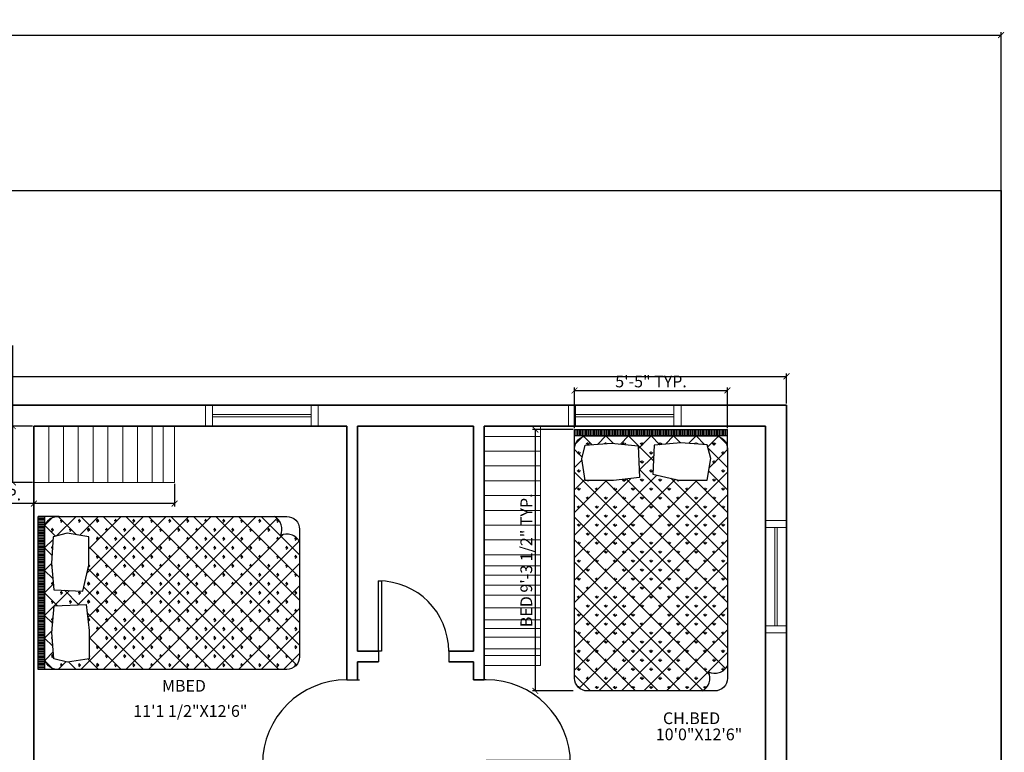
# Model space of a CAD drawing. Units: inches. Extents: x 3283068 to 3284536, y 3240756 to 3241803.
# Tile 19 of 19: x 3283910 to 3284329, y 3241491 to 3241803. Entities that reach past the tile are written whole.
import ezdxf

# ---------------------------------------------------------------- set-up
doc = ezdxf.new("R2010")
doc.units = ezdxf.units.IN
for name, color, linetype, lineweight in [('A-ANNO-DIMS', 2, 'Continuous', 18), ('A-AREA-IDEN', 7, 'Continuous', 18), ('C-PROP', 7, 'Continuous', 25), ('door', 140, 'Continuous', 25), ('furniture', 40, 'Continuous', 18), ('wall', 20, 'Continuous', 35), ('wardrobe', 180, 'Continuous', 18), ('window', 100, 'Continuous', 18)]:
    doc.layers.add(name, color=color, linetype=linetype, lineweight=lineweight)
doc.layers.add('NOI THAT', color=42, linetype='Continuous')
doc.styles.get("Standard").update_dxf_attribs({"font": 'arial.ttf'})
doc.dimstyles.new('ISO-25', dxfattribs={"dimtxt": 5, "dimasz": 2.5, "dimexe": 1.25, "dimexo": 0.625, "dimtad": 1, "dimlunit": 4, "dimtxsty": 'Standard', "dimblk": 'ARCHTICK', "dimcen": 2.5, "dimadec": 0, "dimazin": 0, "dimtfac": 1, "dimtmove": 0, "dimatfit": 3, "dimfxl": 1, "dimarcsym": 0})

# ---------------------------------------------------------------- blocks, each defined once
blk = doc.blocks.new('*U5')
for p, q in [((-40, 0), (-40, 6)), ((0, 0), (0, 6))]:
    blk.add_line(p, q)
blk.add_lwpolyline([(0, 0), (0, -40), (-1.75, -40), (-1.75, 0)], close=True)
blk.add_arc((0, 0), 40, 180, 270)
blk = doc.blocks.new('*U6')
for p, q in [((0, 0), (0, -6)), ((-40, 0), (-40, -6))]:
    blk.add_line(p, q)
blk.add_lwpolyline([(0, 0), (0, 40), (-1.75, 40), (-1.75, 0)], close=True)
blk.add_arc((0, 0), 40, 90, 180)
blk = doc.blocks.new('*U4')
for p, q in [((-40, 0), (-40, 6)), ((0, 0), (0, 6))]:
    blk.add_line(p, q)
blk.add_lwpolyline([(0, 0), (0, -40), (-1.75, -40), (-1.75, 0)], close=True)
blk.add_arc((0, 0), 40, 180, 270)
blk = doc.blocks.new('*X15')
at = {"color": 0}
for p, q in [((-424.3, 0), (-424.3, 0)), ((-424.3, 0), (-424.3, 0)), ((-141.4, 0), (-141.4, 0)), ((-495.1, -70.6), (-508.2, -57.5)), ((-495, -70.6), (-495, -52)), ((-494.9, -70.6), (-481.7, -57.5)), ((-363.4, -60.9), (-366.8, -57.5)), ((-353.6, -60.2), (-353.6, -52)), ((-342.2, -59.3), (-340.3, -57.5)), ((-282.8, 0), (-282.8, 0)), ((-282.8, 0), (-282.8, 0)), ((-217.5, -65.3), (-225.4, -57.5)), ((-212.1, -65.8), (-212.1, -52)), ((-207.7, -66.2), (-198.9, -57.5)), ((-70.7, -70.7), (-84, -57.5)), ((-70.7, -70.7), (-70.7, -52)), ((-70.7, -70.7), (-57.5, -57.5)), ((68.3, -68.3), (57.5, -57.5)), ((70.7, -68.1), (70.7, -52)), ((73.6, -67.8), (84, -57.5)), ((212.1, -55), (212.1, -52)), ((282.8, 0), (282.8, 0)), ((344.1, -61.2), (340.3, -57.5)), ((353.6, -61.9), (353.6, -52)), ((361.7, -62.5), (366.8, -57.5)), ((424.3, 0), (424.3, 0)), ((495, -70.7), (481.7, -57.5)), ((495, -70.7), (495, -52)), ((495, -70.7), (508.2, -57.5)), ((-565.7, -141.4), (-578.9, -128.2)), ((-565.7, -141.4), (-565.7, -122.7)), ((-565.7, -141.4), (-552.4, -128.2)), ((0, -141.4), (-13.3, -128.2)), ((0, -141.4), (0, -122.7)), ((0, -141.4), (13.3, -128.2)), ((565.7, -141.4), (552.4, -128.2)), ((565.7, -141.4), (565.7, -122.7)), ((565.7, -141.4), (578.9, -128.2)), ((-70.7, -212.1), (-84, -198.9)), ((-70.7, -212.1), (-70.7, -193.4)), ((-70.7, -212.1), (-57.5, -198.9)), ((495, -212.1), (481.7, -198.9)), ((495, -212.1), (495, -193.4)), ((495, -212.1), (508.2, -198.9)), ((-565.7, -282.8), (-578.9, -269.6)), ((-565.7, -282.8), (-565.7, -264.1)), ((-565.7, -282.8), (-552.4, -269.6)), ((0, -282.8), (-13.3, -269.6)), ((0, -282.8), (0, -264.1)), ((0, -282.8), (13.3, -269.6)), ((565.7, -282.8), (552.4, -269.6)), ((565.7, -282.8), (565.7, -264.1)), ((565.7, -282.8), (578.9, -269.6)), ((-495, -353.6), (-499, -349.5)), ((-495, -353.6), (-495, -349.5)), ((-495, -353.6), (-491, -349.5)), ((-353.6, -353.6), (-357.6, -349.5)), ((-353.6, -353.6), (-353.6, -349.5)), ((-353.6, -353.6), (-349.5, -349.5)), ((-212.1, -353.6), (-224, -341.7)), ((-212.1, -353.6), (-212.1, -340.3)), ((-212.1, -353.6), (-198.9, -340.3)), ((-70.7, -353.6), (-84, -340.3)), ((-70.7, -353.6), (-70.7, -334.8)), ((-70.7, -353.6), (-57.5, -340.3)), ((70.7, -353.6), (57.5, -340.3)), ((70.7, -353.6), (70.7, -334.8)), ((70.7, -353.6), (84, -340.3)), ((212.1, -353.6), (200.4, -341.8)), ((212.1, -353.6), (212.1, -344.4)), ((212.1, -353.6), (220, -345.7)), ((353.6, -353.6), (345.7, -345.7)), ((353.6, -353.6), (353.6, -345.7)), ((353.6, -353.6), (361.4, -345.7)), ((495, -353.6), (481.7, -340.3)), ((495, -353.6), (495, -334.8)), ((495, -353.6), (508.2, -340.3)), ((-565.7, -424.3), (-578.9, -411)), ((-565.7, -424.3), (-565.7, -405.5)), ((-565.7, -424.3), (-552.4, -411)), ((-424.3, -424.3), (-437.5, -411)), ((-424.3, -424.3), (-424.3, -405.5)), ((-424.3, -424.3), (-411, -411)), ((-282.8, -424.3), (-296.1, -411)), ((-282.8, -424.3), (-282.8, -405.5)), ((-282.8, -424.3), (-269.6, -411)), ((-141.4, -424.3), (-154.7, -411)), ((-141.4, -424.3), (-141.4, -405.5)), ((-141.4, -424.3), (-128.2, -411)), ((0, -424.3), (-13.3, -411)), ((0, -424.3), (0, -405.5)), ((0, -424.3), (13.3, -411)), ((141.4, -424.3), (128.2, -411)), ((141.4, -424.3), (141.4, -405.5)), ((141.4, -424.3), (154.7, -411)), ((282.8, -424.3), (269.6, -411)), ((282.8, -424.3), (282.8, -405.5)), ((282.8, -424.3), (296.1, -411)), ((424.3, -424.3), (411, -411)), ((424.3, -424.3), (424.3, -405.5)), ((424.3, -424.3), (437.5, -411)), ((565.7, -424.3), (552.4, -411)), ((565.7, -424.3), (565.7, -405.5)), ((565.7, -424.3), (578.9, -411)), ((-495, -495), (-508.2, -481.7)), ((-495, -495), (-495, -476.2)), ((-495, -495), (-481.7, -481.7)), ((-353.6, -495), (-366.8, -481.7)), ((-353.6, -495), (-353.6, -476.2)), ((-353.6, -495), (-340.3, -481.7)), ((-212.1, -495), (-225.4, -481.7)), ((-212.1, -495), (-212.1, -476.2)), ((-212.1, -495), (-198.9, -481.7)), ((-70.7, -495), (-84, -481.7)), ((-70.7, -495), (-70.7, -476.2)), ((-70.7, -495), (-57.5, -481.7)), ((70.7, -495), (57.5, -481.7)), ((70.7, -495), (70.7, -476.2)), ((70.7, -495), (84, -481.7)), ((212.1, -495), (198.9, -481.7)), ((212.1, -495), (212.1, -476.2)), ((212.1, -495), (225.4, -481.7)), ((353.6, -495), (340.3, -481.7)), ((353.6, -495), (353.6, -476.2)), ((353.6, -495), (366.8, -481.7)), ((495, -495), (481.7, -481.7)), ((495, -495), (495, -476.2)), ((495, -495), (508.2, -481.7)), ((-565.7, -565.7), (-578.9, -552.4)), ((-565.7, -565.7), (-565.7, -546.9)), ((-565.7, -565.7), (-552.4, -552.4)), ((-495, -636.4), (-495, -617.6)), ((-424.3, -565.7), (-437.5, -552.4)), ((-424.3, -565.7), (-424.3, -546.9)), ((-424.3, -565.7), (-411, -552.4)), ((-353.6, -636.4), (-353.6, -617.6)), ((-282.8, -565.7), (-296.1, -552.4)), ((-282.8, -565.7), (-282.8, -546.9)), ((-282.8, -565.7), (-269.6, -552.4)), ((-212.1, -636.4), (-212.1, -617.6)), ((-141.4, -565.7), (-154.7, -552.4)), ((-141.4, -565.7), (-141.4, -546.9)), ((-141.4, -565.7), (-128.2, -552.4)), ((-70.7, -636.4), (-70.7, -617.6)), ((0, -565.7), (-13.3, -552.4)), ((0, -565.7), (0, -546.9)), ((0, -565.7), (13.3, -552.4)), ((70.7, -636.4), (70.7, -617.6)), ((141.4, -565.7), (128.2, -552.4)), ((141.4, -565.7), (141.4, -546.9)), ((141.4, -565.7), (154.7, -552.4)), ((212.1, -636.4), (212.1, -617.6)), ((282.8, -565.7), (269.6, -552.4)), ((282.8, -565.7), (282.8, -546.9)), ((282.8, -565.7), (296.1, -552.4)), ((353.6, -636.4), (353.6, -617.6)), ((424.3, -565.7), (411, -552.4)), ((424.3, -565.7), (424.3, -546.9)), ((424.3, -565.7), (437.5, -552.4)), ((495, -636.4), (495, -617.6)), ((565.7, -565.7), (552.4, -552.4)), ((565.7, -565.7), (565.7, -546.9)), ((565.7, -565.7), (578.9, -552.4)), ((-565.7, -707.1), (-578.9, -693.8)), ((-565.7, -707.1), (-565.7, -688.4)), ((-565.7, -707.1), (-552.4, -693.8)), ((-495, -636.4), (-508.2, -623.1)), ((-495, -636.4), (-481.7, -623.1)), ((-424.3, -707.1), (-437.5, -693.8)), ((-424.3, -707.1), (-424.3, -688.4)), ((-424.3, -707.1), (-411, -693.8)), ((-353.6, -636.4), (-366.8, -623.1)), ((-353.6, -636.4), (-340.3, -623.1)), ((-282.8, -707.1), (-296.1, -693.8)), ((-282.8, -707.1), (-282.8, -688.4)), ((-282.8, -707.1), (-269.6, -693.8)), ((-212.1, -636.4), (-225.4, -623.1)), ((-212.1, -636.4), (-198.9, -623.1)), ((-141.4, -707.1), (-154.7, -693.8)), ((-141.4, -707.1), (-141.4, -688.4)), ((-141.4, -707.1), (-128.2, -693.8)), ((-70.7, -636.4), (-84, -623.1)), ((-70.7, -636.4), (-57.5, -623.1)), ((0, -707.1), (-13.3, -693.8)), ((0, -707.1), (0, -688.4)), ((0, -707.1), (13.3, -693.8)), ((70.7, -636.4), (57.5, -623.1)), ((70.7, -636.4), (84, -623.1)), ((141.4, -707.1), (128.2, -693.8)), ((141.4, -707.1), (141.4, -688.4)), ((141.4, -707.1), (154.7, -693.8)), ((212.1, -636.4), (198.9, -623.1)), ((212.1, -636.4), (225.4, -623.1)), ((282.8, -707.1), (269.6, -693.8)), ((282.8, -707.1), (282.8, -688.4)), ((282.8, -707.1), (296.1, -693.8)), ((353.6, -636.4), (340.3, -623.1)), ((353.6, -636.4), (366.8, -623.1)), ((424.3, -707.1), (411, -693.8)), ((424.3, -707.1), (424.3, -688.4)), ((424.3, -707.1), (437.5, -693.8)), ((495, -636.4), (481.7, -623.1)), ((495, -636.4), (508.2, -623.1)), ((565.7, -707.1), (552.4, -693.8)), ((565.7, -707.1), (565.7, -688.4)), ((565.7, -707.1), (578.9, -693.8)), ((-495, -777.8), (-508.2, -764.6)), ((-495, -777.8), (-495, -759.1)), ((-495, -777.8), (-481.7, -764.6)), ((-353.6, -777.8), (-366.8, -764.6)), ((-353.6, -777.8), (-353.6, -759.1)), ((-353.6, -777.8), (-340.3, -764.6)), ((-212.1, -777.8), (-225.4, -764.6)), ((-212.1, -777.8), (-212.1, -759.1)), ((-212.1, -777.8), (-198.9, -764.6)), ((-70.7, -777.8), (-84, -764.6)), ((-70.7, -777.8), (-70.7, -759.1)), ((-70.7, -777.8), (-57.5, -764.6)), ((70.7, -777.8), (57.5, -764.6)), ((70.7, -777.8), (70.7, -759.1)), ((70.7, -777.8), (84, -764.6)), ((212.1, -777.8), (198.9, -764.6)), ((212.1, -777.8), (212.1, -759.1)), ((212.1, -777.8), (225.4, -764.6)), ((353.6, -777.8), (340.3, -764.6)), ((353.6, -777.8), (353.6, -759.1)), ((353.6, -777.8), (366.8, -764.6)), ((495, -777.8), (481.7, -764.6)), ((495, -777.8), (495, -759.1)), ((495, -777.8), (508.2, -764.6)), ((-565.7, -848.5), (-578.9, -835.3)), ((-565.7, -848.5), (-565.7, -829.8)), ((-565.7, -848.5), (-552.4, -835.3)), ((-424.3, -848.5), (-437.5, -835.3)), ((-424.3, -848.5), (-424.3, -829.8)), ((-424.3, -848.5), (-411, -835.3)), ((-282.8, -848.5), (-296.1, -835.3)), ((-282.8, -848.5), (-282.8, -829.8)), ((-282.8, -848.5), (-269.6, -835.3)), ((-141.4, -848.5), (-154.7, -835.3)), ((-141.4, -848.5), (-141.4, -829.8)), ((-141.4, -848.5), (-128.2, -835.3)), ((0, -848.5), (-13.3, -835.3)), ((0, -848.5), (0, -829.8)), ((0, -848.5), (13.3, -835.3)), ((141.4, -848.5), (128.2, -835.3)), ((141.4, -848.5), (141.4, -829.8)), ((141.4, -848.5), (154.7, -835.3)), ((282.8, -848.5), (269.6, -835.3)), ((282.8, -848.5), (282.8, -829.8)), ((282.8, -848.5), (296.1, -835.3)), ((424.3, -848.5), (411, -835.3)), ((424.3, -848.5), (424.3, -829.8)), ((424.3, -848.5), (437.5, -835.3)), ((565.7, -848.5), (552.4, -835.3)), ((565.7, -848.5), (565.7, -829.8)), ((565.7, -848.5), (578.9, -835.3)), ((-495, -919.2), (-508.2, -906)), ((-495, -919.2), (-495, -900.5)), ((-495, -919.2), (-481.7, -906)), ((-353.6, -919.2), (-366.8, -906)), ((-353.6, -919.2), (-353.6, -900.5)), ((-353.6, -919.2), (-340.3, -906)), ((-212.1, -919.2), (-225.4, -906)), ((-212.1, -919.2), (-212.1, -900.5)), ((-212.1, -919.2), (-198.9, -906)), ((-70.7, -919.2), (-84, -906)), ((-70.7, -919.2), (-70.7, -900.5)), ((-70.7, -919.2), (-57.5, -906)), ((70.7, -919.2), (57.5, -906)), ((70.7, -919.2), (70.7, -900.5)), ((70.7, -919.2), (84, -906)), ((212.1, -919.2), (198.9, -906)), ((212.1, -919.2), (212.1, -900.5)), ((212.1, -919.2), (225.4, -906)), ((353.6, -919.2), (340.3, -906)), ((353.6, -919.2), (353.6, -900.5)), ((353.6, -919.2), (366.8, -906)), ((495, -919.2), (481.7, -906)), ((495, -919.2), (495, -900.5)), ((495, -919.2), (508.2, -906)), ((-565.7, -989.9), (-578.9, -976.7)), ((-565.7, -989.9), (-565.7, -971.2)), ((-565.7, -989.9), (-552.4, -976.7)), ((-424.3, -989.9), (-437.5, -976.7)), ((-424.3, -989.9), (-424.3, -971.2)), ((-424.3, -989.9), (-411, -976.7)), ((-282.8, -989.9), (-296.1, -976.7)), ((-282.8, -989.9), (-282.8, -971.2)), ((-282.8, -989.9), (-269.6, -976.7)), ((-141.4, -989.9), (-154.7, -976.7)), ((-141.4, -989.9), (-141.4, -971.2)), ((-141.4, -989.9), (-128.2, -976.7)), ((0, -989.9), (-13.3, -976.7)), ((0, -989.9), (0, -971.2)), ((0, -989.9), (13.3, -976.7)), ((141.4, -989.9), (128.2, -976.7)), ((141.4, -989.9), (141.4, -971.2)), ((141.4, -989.9), (154.7, -976.7)), ((282.8, -989.9), (269.6, -976.7)), ((282.8, -989.9), (282.8, -971.2)), ((282.8, -989.9), (296.1, -976.7)), ((424.3, -989.9), (411, -976.7)), ((424.3, -989.9), (424.3, -971.2)), ((424.3, -989.9), (437.5, -976.7)), ((565.7, -989.9), (552.4, -976.7)), ((565.7, -989.9), (565.7, -971.2)), ((565.7, -989.9), (578.9, -976.7)), ((-495, -1060.7), (-508.2, -1047.4)), ((-495, -1060.7), (-495, -1041.9)), ((-495, -1060.7), (-481.7, -1047.4)), ((-353.6, -1060.7), (-366.8, -1047.4)), ((-353.6, -1060.7), (-353.6, -1041.9)), ((-353.6, -1060.7), (-340.3, -1047.4)), ((-212.1, -1060.7), (-225.4, -1047.4)), ((-212.1, -1060.7), (-212.1, -1041.9)), ((-212.1, -1060.7), (-198.9, -1047.4)), ((-70.7, -1060.7), (-84, -1047.4)), ((-70.7, -1060.7), (-70.7, -1041.9)), ((-70.7, -1060.7), (-57.5, -1047.4)), ((70.7, -1060.7), (57.5, -1047.4)), ((70.7, -1060.7), (70.7, -1041.9)), ((70.7, -1060.7), (84, -1047.4)), ((212.1, -1060.7), (198.9, -1047.4)), ((212.1, -1060.7), (212.1, -1041.9)), ((212.1, -1060.7), (225.4, -1047.4)), ((353.6, -1060.7), (340.3, -1047.4)), ((353.6, -1060.7), (353.6, -1041.9)), ((353.6, -1060.7), (366.8, -1047.4)), ((495, -1060.7), (481.7, -1047.4)), ((495, -1060.7), (495, -1041.9)), ((495, -1060.7), (508.2, -1047.4)), ((-565.7, -1131.4), (-578.9, -1118.1)), ((-565.7, -1131.4), (-565.7, -1112.6)), ((-565.7, -1131.4), (-552.4, -1118.1)), ((-424.3, -1131.4), (-437.5, -1118.1)), ((-424.3, -1131.4), (-424.3, -1112.6)), ((-424.3, -1131.4), (-411, -1118.1)), ((-282.8, -1131.4), (-296.1, -1118.1)), ((-282.8, -1131.4), (-282.8, -1112.6)), ((-282.8, -1131.4), (-269.6, -1118.1)), ((-141.4, -1131.4), (-154.7, -1118.1)), ((-141.4, -1131.4), (-141.4, -1112.6)), ((-141.4, -1131.4), (-128.2, -1118.1)), ((0, -1131.4), (-13.3, -1118.1)), ((0, -1131.4), (0, -1112.6)), ((0, -1131.4), (13.3, -1118.1)), ((141.4, -1131.4), (128.2, -1118.1)), ((141.4, -1131.4), (141.4, -1112.6)), ((141.4, -1131.4), (154.7, -1118.1)), ((282.8, -1131.4), (269.6, -1118.1)), ((282.8, -1131.4), (282.8, -1112.6)), ((282.8, -1131.4), (296.1, -1118.1)), ((424.3, -1131.4), (411, -1118.1)), ((424.3, -1131.4), (424.3, -1112.6)), ((424.3, -1131.4), (437.5, -1118.1)), ((565.7, -1131.4), (552.4, -1118.1)), ((565.7, -1131.4), (565.7, -1112.6)), ((565.7, -1131.4), (578.9, -1118.1)), ((-495, -1202.1), (-508.2, -1188.8)), ((-495, -1202.1), (-495, -1183.3)), ((-495, -1202.1), (-481.7, -1188.8)), ((-353.6, -1202.1), (-366.8, -1188.8)), ((-353.6, -1202.1), (-353.6, -1183.3)), ((-353.6, -1202.1), (-340.3, -1188.8)), ((-212.1, -1202.1), (-225.4, -1188.8)), ((-212.1, -1202.1), (-212.1, -1183.3)), ((-212.1, -1202.1), (-198.9, -1188.8)), ((-70.7, -1202.1), (-84, -1188.8)), ((-70.7, -1202.1), (-70.7, -1183.3)), ((-70.7, -1202.1), (-57.5, -1188.8)), ((70.7, -1202.1), (57.5, -1188.8)), ((70.7, -1202.1), (70.7, -1183.3)), ((70.7, -1202.1), (84, -1188.8)), ((212.1, -1202.1), (198.9, -1188.8)), ((212.1, -1202.1), (212.1, -1183.3)), ((212.1, -1202.1), (225.4, -1188.8)), ((353.6, -1202.1), (340.3, -1188.8)), ((353.6, -1202.1), (353.6, -1183.3)), ((353.6, -1202.1), (366.8, -1188.8)), ((495, -1202.1), (481.7, -1188.8)), ((495, -1202.1), (495, -1183.3)), ((495, -1202.1), (508.2, -1188.8)), ((-565.7, -1272.8), (-578.9, -1259.5)), ((-565.7, -1272.8), (-565.7, -1254)), ((-565.7, -1272.8), (-552.4, -1259.5)), ((-424.3, -1272.8), (-437.5, -1259.5)), ((-424.3, -1272.8), (-424.3, -1254)), ((-424.3, -1272.8), (-411, -1259.5)), ((-282.8, -1272.8), (-296.1, -1259.5)), ((-282.8, -1272.8), (-282.8, -1254)), ((-282.8, -1272.8), (-269.6, -1259.5)), ((-141.4, -1272.8), (-154.7, -1259.5)), ((-141.4, -1272.8), (-141.4, -1254)), ((-141.4, -1272.8), (-128.2, -1259.5)), ((0, -1272.8), (-13.3, -1259.5)), ((0, -1272.8), (0, -1254)), ((0, -1272.8), (13.3, -1259.5)), ((141.4, -1272.8), (128.2, -1259.5)), ((141.4, -1272.8), (141.4, -1254)), ((141.4, -1272.8), (154.7, -1259.5)), ((282.8, -1272.8), (269.6, -1259.5)), ((282.8, -1272.8), (282.8, -1254)), ((282.8, -1272.8), (296.1, -1259.5)), ((424.3, -1272.8), (411, -1259.5)), ((424.3, -1272.8), (424.3, -1254)), ((424.3, -1272.8), (437.5, -1259.5)), ((565.7, -1272.8), (552.4, -1259.5)), ((565.7, -1272.8), (565.7, -1254)), ((565.7, -1272.8), (578.9, -1259.5)), ((-495, -1343.5), (-508.2, -1330.2)), ((-495, -1343.5), (-495, -1324.8)), ((-495, -1343.5), (-481.7, -1330.2)), ((-353.6, -1343.5), (-366.8, -1330.2)), ((-353.6, -1343.5), (-353.6, -1324.8)), ((-353.6, -1343.5), (-340.3, -1330.2)), ((-212.1, -1343.5), (-225.4, -1330.2)), ((-212.1, -1343.5), (-212.1, -1324.8)), ((-212.1, -1343.5), (-198.9, -1330.2)), ((-70.7, -1343.5), (-84, -1330.2)), ((-70.7, -1343.5), (-70.7, -1324.8)), ((-70.7, -1343.5), (-57.5, -1330.2)), ((70.7, -1343.5), (57.5, -1330.2)), ((70.7, -1343.5), (70.7, -1324.8)), ((70.7, -1343.5), (84, -1330.2)), ((212.1, -1343.5), (198.9, -1330.2)), ((212.1, -1343.5), (212.1, -1324.8)), ((212.1, -1343.5), (225.4, -1330.2)), ((353.6, -1343.5), (340.3, -1330.2)), ((353.6, -1343.5), (353.6, -1324.8)), ((353.6, -1343.5), (366.8, -1330.2)), ((495, -1343.5), (481.7, -1330.2)), ((495, -1343.5), (495, -1324.8)), ((495, -1343.5), (508.2, -1330.2)), ((-565.7, -1414.2), (-578.9, -1401)), ((-565.7, -1414.2), (-565.7, -1395.5)), ((-565.7, -1414.2), (-552.4, -1401)), ((-495, -1484.9), (-495, -1466.2)), ((-424.3, -1414.2), (-437.5, -1401)), ((-424.3, -1414.2), (-424.3, -1395.5)), ((-424.3, -1414.2), (-411, -1401)), ((-353.6, -1484.9), (-353.6, -1466.2)), ((-282.8, -1414.2), (-296.1, -1401)), ((-282.8, -1414.2), (-282.8, -1395.5)), ((-282.8, -1414.2), (-269.6, -1401)), ((-212.1, -1484.9), (-212.1, -1466.2)), ((-141.4, -1414.2), (-154.7, -1401)), ((-141.4, -1414.2), (-141.4, -1395.5)), ((-141.4, -1414.2), (-128.2, -1401)), ((-70.7, -1484.9), (-70.7, -1466.2)), ((0, -1414.2), (-13.3, -1401)), ((0, -1414.2), (0, -1395.5)), ((0, -1414.2), (13.3, -1401)), ((70.7, -1484.9), (70.7, -1466.2)), ((141.4, -1414.2), (128.2, -1401)), ((141.4, -1414.2), (141.4, -1395.5)), ((141.4, -1414.2), (154.7, -1401)), ((212.1, -1484.9), (212.1, -1466.2)), ((282.8, -1414.2), (269.6, -1401)), ((282.8, -1414.2), (282.8, -1395.5)), ((282.8, -1414.2), (296.1, -1401)), ((353.6, -1484.9), (353.6, -1466.2)), ((424.3, -1414.2), (411, -1401)), ((424.3, -1414.2), (424.3, -1395.5)), ((424.3, -1414.2), (437.5, -1401)), ((495, -1484.9), (495, -1466.2)), ((565.7, -1414.2), (552.4, -1401)), ((565.7, -1414.2), (565.7, -1395.5)), ((565.7, -1414.2), (578.9, -1401)), ((-565.7, -1555.6), (-578.9, -1542.4)), ((-565.7, -1555.6), (-565.7, -1536.9)), ((-565.7, -1555.6), (-552.4, -1542.4)), ((-495, -1484.9), (-508.2, -1471.7)), ((-495, -1484.9), (-481.7, -1471.7)), ((-424.3, -1555.6), (-437.5, -1542.4)), ((-424.3, -1555.6), (-424.3, -1536.9)), ((-424.3, -1555.6), (-411, -1542.4)), ((-353.6, -1484.9), (-366.8, -1471.7)), ((-353.6, -1484.9), (-340.3, -1471.7)), ((-282.8, -1555.6), (-296.1, -1542.4)), ((-282.8, -1555.6), (-282.8, -1536.9)), ((-282.8, -1555.6), (-269.6, -1542.4)), ((-212.1, -1484.9), (-225.4, -1471.7)), ((-212.1, -1484.9), (-198.9, -1471.7)), ((-141.4, -1555.6), (-154.7, -1542.4)), ((-141.4, -1555.6), (-141.4, -1536.9)), ((-141.4, -1555.6), (-128.2, -1542.4)), ((-70.7, -1484.9), (-84, -1471.7)), ((-70.7, -1484.9), (-57.5, -1471.7)), ((0, -1555.6), (-13.3, -1542.4)), ((0, -1555.6), (0, -1536.9)), ((0, -1555.6), (13.3, -1542.4)), ((70.7, -1484.9), (57.5, -1471.7)), ((70.7, -1484.9), (84, -1471.7)), ((141.4, -1555.6), (128.2, -1542.4)), ((141.4, -1555.6), (141.4, -1536.9)), ((141.4, -1555.6), (154.7, -1542.4)), ((212.1, -1484.9), (198.9, -1471.7)), ((212.1, -1484.9), (225.4, -1471.7)), ((282.8, -1555.6), (269.6, -1542.4)), ((282.8, -1555.6), (282.8, -1536.9)), ((282.8, -1555.6), (296.1, -1542.4)), ((353.6, -1484.9), (340.3, -1471.7)), ((353.6, -1484.9), (366.8, -1471.7)), ((424.3, -1555.6), (411, -1542.4)), ((424.3, -1555.6), (424.3, -1536.9)), ((424.3, -1555.6), (437.5, -1542.4)), ((495, -1484.9), (481.7, -1471.7)), ((495, -1484.9), (508.2, -1471.7)), ((565.7, -1555.6), (552.4, -1542.4)), ((565.7, -1555.6), (565.7, -1536.9)), ((565.7, -1555.6), (578.9, -1542.4)), ((-495, -1626.3), (-508.2, -1613.1)), ((-495, -1626.3), (-495, -1607.6)), ((-495, -1626.3), (-481.7, -1613.1)), ((-353.6, -1626.3), (-366.8, -1613.1)), ((-353.6, -1626.3), (-353.6, -1607.6)), ((-353.6, -1626.3), (-340.3, -1613.1)), ((-212.1, -1626.3), (-225.4, -1613.1)), ((-212.1, -1626.3), (-212.1, -1607.6)), ((-212.1, -1626.3), (-198.9, -1613.1)), ((-70.7, -1626.3), (-84, -1613.1)), ((-70.7, -1626.3), (-70.7, -1607.6)), ((-70.7, -1626.3), (-57.5, -1613.1)), ((70.7, -1626.3), (57.5, -1613.1)), ((70.7, -1626.3), (70.7, -1607.6)), ((70.7, -1626.3), (84, -1613.1)), ((212.1, -1626.3), (198.9, -1613.1)), ((212.1, -1626.3), (212.1, -1607.6)), ((212.1, -1626.3), (225.4, -1613.1)), ((353.6, -1626.3), (340.3, -1613.1)), ((353.6, -1626.3), (353.6, -1607.6)), ((353.6, -1626.3), (366.8, -1613.1)), ((495, -1626.3), (481.7, -1613.1)), ((495, -1626.3), (495, -1607.6)), ((495, -1626.3), (508.2, -1613.1)), ((-565.7, -1697.1), (-578.9, -1683.8)), ((-565.7, -1697.1), (-565.7, -1678.3)), ((-565.7, -1697.1), (-552.4, -1683.8)), ((-424.3, -1697.1), (-437.5, -1683.8)), ((-424.3, -1697.1), (-424.3, -1678.3)), ((-424.3, -1697.1), (-411, -1683.8)), ((-282.8, -1697.1), (-296.1, -1683.8)), ((-282.8, -1697.1), (-282.8, -1678.3)), ((-282.8, -1697.1), (-269.6, -1683.8)), ((-141.4, -1697.1), (-154.7, -1683.8)), ((-141.4, -1697.1), (-141.4, -1678.3)), ((-141.4, -1697.1), (-128.2, -1683.8)), ((0, -1697.1), (-13.3, -1683.8)), ((0, -1697.1), (0, -1678.3)), ((0, -1697.1), (13.3, -1683.8)), ((141.4, -1697.1), (128.2, -1683.8)), ((141.4, -1697.1), (141.4, -1678.3)), ((141.4, -1697.1), (154.7, -1683.8)), ((282.8, -1697.1), (269.6, -1683.8)), ((282.8, -1697.1), (282.8, -1678.3)), ((282.8, -1697.1), (296.1, -1683.8)), ((424.3, -1697.1), (411, -1683.8)), ((424.3, -1697.1), (424.3, -1678.3)), ((424.3, -1697.1), (437.5, -1683.8)), ((565.7, -1697.1), (552.4, -1683.8)), ((565.7, -1697.1), (565.7, -1678.3)), ((565.7, -1697.1), (578.9, -1683.8)), ((-495, -1767.8), (-508.2, -1754.5)), ((-495, -1767.8), (-495, -1749)), ((-495, -1767.8), (-481.7, -1754.5)), ((-353.6, -1767.8), (-366.8, -1754.5)), ((-353.6, -1767.8), (-353.6, -1749)), ((-353.6, -1767.8), (-340.3, -1754.5)), ((-212.1, -1767.8), (-225.4, -1754.5)), ((-212.1, -1767.8), (-212.1, -1749)), ((-212.1, -1767.8), (-198.9, -1754.5)), ((-70.7, -1767.8), (-84, -1754.5)), ((-70.7, -1767.8), (-70.7, -1749)), ((-70.7, -1767.8), (-57.5, -1754.5)), ((70.7, -1767.8), (57.5, -1754.5)), ((70.7, -1767.8), (70.7, -1749)), ((70.7, -1767.8), (84, -1754.5)), ((212.1, -1767.8), (198.9, -1754.5)), ((212.1, -1767.8), (212.1, -1749)), ((212.1, -1767.8), (225.4, -1754.5)), ((353.6, -1767.8), (340.3, -1754.5)), ((353.6, -1767.8), (353.6, -1749)), ((353.6, -1767.8), (366.8, -1754.5)), ((495, -1767.8), (481.7, -1754.5)), ((495, -1767.8), (495, -1749)), ((495, -1767.8), (508.2, -1754.5)), ((-565.7, -1838.5), (-578.9, -1825.2)), ((-565.7, -1838.5), (-565.7, -1819.7)), ((-565.7, -1838.5), (-552.4, -1825.2)), ((-424.3, -1838.5), (-437.5, -1825.2)), ((-424.3, -1838.5), (-424.3, -1819.7)), ((-424.3, -1838.5), (-411, -1825.2)), ((-282.8, -1838.5), (-296.1, -1825.2)), ((-282.8, -1838.5), (-282.8, -1819.7)), ((-282.8, -1838.5), (-269.6, -1825.2)), ((-141.4, -1838.5), (-154.7, -1825.2)), ((-141.4, -1838.5), (-141.4, -1819.7)), ((-141.4, -1838.5), (-128.2, -1825.2)), ((0, -1838.5), (-13.3, -1825.2)), ((0, -1838.5), (0, -1819.7)), ((0, -1838.5), (13.3, -1825.2)), ((141.4, -1838.5), (128.2, -1825.2)), ((141.4, -1838.5), (141.4, -1819.7)), ((141.4, -1838.5), (154.7, -1825.2)), ((282.8, -1838.5), (269.6, -1825.2)), ((282.8, -1838.5), (282.8, -1819.7)), ((282.8, -1838.5), (296.1, -1825.2)), ((424.3, -1838.5), (411, -1825.2)), ((424.3, -1838.5), (424.3, -1819.7)), ((424.3, -1838.5), (437.5, -1825.2)), ((565.7, -1838.5), (552.4, -1825.2)), ((565.7, -1838.5), (565.7, -1819.7)), ((565.7, -1838.5), (578.9, -1825.2)), ((-495, -1909.2), (-508.2, -1895.9)), ((-495, -1909.2), (-495, -1890.4)), ((-495, -1909.2), (-481.7, -1895.9)), ((-353.6, -1909.2), (-366.8, -1895.9)), ((-353.6, -1909.2), (-353.6, -1890.4)), ((-353.6, -1909.2), (-340.3, -1895.9)), ((-212.1, -1909.2), (-225.4, -1895.9)), ((-212.1, -1909.2), (-212.1, -1890.4)), ((-212.1, -1909.2), (-198.9, -1895.9)), ((-70.7, -1909.2), (-84, -1895.9)), ((-70.7, -1909.2), (-70.7, -1890.4)), ((-70.7, -1909.2), (-57.5, -1895.9)), ((70.7, -1909.2), (57.5, -1895.9)), ((70.7, -1909.2), (70.7, -1890.4)), ((70.7, -1909.2), (84, -1895.9)), ((212.1, -1909.2), (198.9, -1895.9)), ((212.1, -1909.2), (212.1, -1890.4)), ((212.1, -1909.2), (225.4, -1895.9)), ((353.6, -1909.2), (340.3, -1895.9)), ((353.6, -1909.2), (353.6, -1890.4)), ((353.6, -1909.2), (366.8, -1895.9)), ((-565.7, -1975.4), (-565.7, -1961.1)), ((-563.2, -1977.5), (-552.4, -1966.6)), ((-424.3, -1979.9), (-437.5, -1966.6)), ((-424.3, -1979.9), (-424.3, -1961.1)), ((-424.3, -1979.9), (-411, -1966.6)), ((-282.8, -1979.9), (-296.1, -1966.6)), ((-282.8, -1979.9), (-282.8, -1961.1)), ((-282.8, -1979.9), (-269.6, -1966.6)), ((-141.4, -1979.9), (-154.7, -1966.6)), ((-141.4, -1979.9), (-141.4, -1961.1)), ((-141.4, -1979.9), (-128.2, -1966.6)), ((0, -1979.9), (-13.3, -1966.6)), ((0, -1979.9), (0, -1961.1)), ((0, -1979.9), (13.3, -1966.6)), ((141.4, -1979.9), (128.2, -1966.6)), ((141.4, -1979.9), (141.4, -1961.1)), ((141.4, -1979.9), (154.7, -1966.6)), ((282.8, -1979.9), (269.6, -1966.6)), ((282.8, -1979.9), (282.8, -1961.1)), ((282.8, -1979.9), (296.1, -1966.6)), ((424.3, -1979.9), (411, -1966.6)), ((424.3, -1979.9), (424.3, -1961.1)), ((424.3, -1979.9), (437.5, -1966.6))]:
    blk.add_line(p, q, dxfattribs=at)
blk = doc.blocks.new('*X14')
at = {"color": 0}
for p, q in [((-592.6, -62.3), (-537.7, -7.4)), ((-462.1, -68.2), (-526.7, -3.6)), ((-418.5, -65), (-353.6, 0)), ((-295.4, -58.1), (-353.6, 0)), ((-240, -63.3), (-176.8, 0)), ((18.9, -195.7), (-176.8, 0)), ((-99.9, -99.9), (0, 0)), ((68.3, -68.3), (0, 0)), ((112.6, -64.2), (176.8, 0)), ((230.1, -53.3), (176.8, 0)), ((295.9, -57.6), (353.6, 0)), ((420.4, -66.9), (353.6, 0)), ((445.5, -84.9), (526.7, -3.6)), ((592.6, -62.3), (537.7, -7.4)), ((-540.7, -166.4), (-600, -107.1)), ((600, -246.4), (447.8, -94.3)), ((456.5, -250.6), (600, -107.1)), ((-600, -246.4), (-542.7, -189.2)), ((-92.1, -268.9), (21, -155.8)), ((-600, -1483.9), (600, -283.9)), ((600, -1483.9), (-600, -283.9)), ((-600, -953.6), (46, -307.5)), ((600, -953.6), (-92.5, -261.1)), ((600, -423.2), (452.5, -275.7)), ((-600, -776.8), (-157.3, -334.1)), ((-600, -1130.3), (190.7, -339.6)), ((-600, -423.2), (-518.4, -341.7)), ((-600, -1307.1), (361.4, -345.7)), ((-600, -600), (-349.5, -349.5)), ((600, -1307.1), (-357.6, -349.5)), ((600, -1130.3), (-192.3, -338.1)), ((600, -776.8), (154.9, -331.7)), ((600, -600), (345.7, -345.7)), ((-600, -1660.7), (600, -460.7)), ((600, -1660.7), (-600, -460.7)), ((-600, -1837.4), (600, -637.4)), ((585.1, -1822.5), (-600, -637.4)), ((458.4, -1872.6), (-600, -814.2)), ((-563.2, -1977.5), (600, -814.2)), ((405.9, -1996.8), (-600, -991)), ((-409, -2000), (600, -991)), ((232.2, -2000), (-600, -1167.8)), ((-232.2, -2000), (600, -1167.8)), ((55.5, -2000), (-600, -1344.5)), ((-55.5, -2000), (600, -1344.5)), ((-121.3, -2000), (-600, -1521.3)), ((121.3, -2000), (600, -1521.3)), ((-298.1, -2000), (-600, -1698.1)), ((298.1, -2000), (600, -1698.1)), ((-474.9, -2000), (-600, -1874.9))]:
    blk.add_line(p, q, dxfattribs=at)
blk = doc.blocks.new('*X16')
at = {"color": 0}
for p, q in [((-587.5, 0), (-587.5, 50)), ((-575, 0), (-575, 50)), ((-562.5, 0), (-562.5, 50)), ((-550, 0), (-550, 50)), ((-537.5, 0), (-537.5, 50)), ((-525, 0), (-525, 50)), ((-512.5, 0), (-512.5, 50)), ((-500, 0), (-500, 50)), ((-487.5, 0), (-487.5, 50)), ((-475, 0), (-475, 50)), ((-462.5, 0), (-462.5, 50)), ((-450, 0), (-450, 50)), ((-437.5, 0), (-437.5, 50)), ((-425, 0), (-425, 50)), ((-412.5, 0), (-412.5, 50)), ((-400, 0), (-400, 50)), ((-387.5, 0), (-387.5, 50)), ((-375, 0), (-375, 50)), ((-362.5, 0), (-362.5, 50)), ((-350, 0), (-350, 50)), ((-337.5, 0), (-337.5, 50)), ((-325, 0), (-325, 50)), ((-312.5, 0), (-312.5, 50)), ((-300, 0), (-300, 50)), ((-287.5, 0), (-287.5, 50)), ((-275, 0), (-275, 50)), ((-262.5, 0), (-262.5, 50)), ((-250, 0), (-250, 50)), ((-237.5, 0), (-237.5, 50)), ((-225, 0), (-225, 50)), ((-212.5, 0), (-212.5, 50)), ((-200, 0), (-200, 50)), ((-187.5, 0), (-187.5, 50)), ((-175, 0), (-175, 50)), ((-162.5, 0), (-162.5, 50)), ((-150, 0), (-150, 50)), ((-137.5, 0), (-137.5, 50)), ((-125, 0), (-125, 50)), ((-112.5, 0), (-112.5, 50)), ((-100, 0), (-100, 50)), ((-87.5, 0), (-87.5, 50)), ((-75, 0), (-75, 50)), ((-62.5, 0), (-62.5, 50)), ((-50, 0), (-50, 50)), ((-37.5, 0), (-37.5, 50)), ((-25, 0), (-25, 50)), ((-12.5, 0), (-12.5, 50)), ((0, 0), (0, 50)), ((12.5, 0), (12.5, 50)), ((25, 0), (25, 50)), ((37.5, 0), (37.5, 50)), ((50, 0), (50, 50)), ((62.5, 0), (62.5, 50)), ((75, 0), (75, 50)), ((87.5, 0), (87.5, 50)), ((100, 0), (100, 50)), ((112.5, 0), (112.5, 50)), ((125, 0), (125, 50)), ((137.5, 0), (137.5, 50)), ((150, 0), (150, 50)), ((162.5, 0), (162.5, 50)), ((175, 0), (175, 50)), ((187.5, 0), (187.5, 50)), ((200, 0), (200, 50)), ((212.5, 0), (212.5, 50)), ((225, 0), (225, 50)), ((237.5, 0), (237.5, 50)), ((250, 0), (250, 50)), ((262.5, 0), (262.5, 50)), ((275, 0), (275, 50)), ((287.5, 0), (287.5, 50)), ((300, 0), (300, 50)), ((312.5, 0), (312.5, 50)), ((325, 0), (325, 50)), ((337.5, 0), (337.5, 50)), ((350, 0), (350, 50)), ((362.5, 0), (362.5, 50)), ((375, 0), (375, 50)), ((387.5, 0), (387.5, 50)), ((400, 0), (400, 50)), ((412.5, 0), (412.5, 50)), ((425, 0), (425, 50)), ((437.5, 0), (437.5, 50)), ((450, 0), (450, 50)), ((462.5, 0), (462.5, 50)), ((475, 0), (475, 50)), ((487.5, 0), (487.5, 50)), ((500, 0), (500, 50)), ((512.5, 0), (512.5, 50)), ((525, 0), (525, 50)), ((537.5, 0), (537.5, 50)), ((550, 0), (550, 50)), ((562.5, 0), (562.5, 50)), ((575, 0), (575, 50)), ((587.5, 0), (587.5, 50))]:
    blk.add_line(p, q, dxfattribs=at)
blk = doc.blocks.new('A$C5BFD579E')
at = {"layer": 'NOI THAT'}
for p, q in [((0, 2050), (1200, 2050)), ((0, 1885.1), (0, 2050)), ((1200, 1885.1), (1200, 2050))]:
    blk.add_line(p, q, dxfattribs=at)
blk.add_lwpolyline([(100, 2000), (1100, 2000, -0.414214), (1200, 1900), (1200, 100, -0.414214), (1100, 0), (100, 0, -0.414214), (0, 100), (0, 1900, -0.414214)], format="xyb", close=True, dxfattribs=at)
blk.add_lwpolyline([(1200, 2000), (0, 2000)], dxfattribs=at)
for points in [[(290.9, 1943.1), (499, 1923.9), (510.6, 1673.6), (306.3, 1650.5), (82.8, 1650.5), (55.8, 1819.9), (82.8, 1927.7)], [(833.3, 1947), (625.2, 1927.7), (613.6, 1699.6), (817.9, 1654.3), (1041.4, 1654.3), (1068.3, 1823.8), (1041.4, 1931.6)]]:
    blk.add_lwpolyline(points, close=True, dxfattribs=at)
for centre, start, end in [((1100, 250), 243.43495, 333.43495), ((950, 100), 296.56505, 26.56505)]:
    blk.add_arc(centre, 111.8, start, end, dxfattribs=at)
for name in ['*X16', '*X14', '*X15']:
    blk.add_blockref(name, (600, 2000), dxfattribs=at)
blk = doc.blocks.new('_ArchTick')
at = {"color": 0, "linetype": 'ByBlock', "const_width": 0.15}
blk.add_lwpolyline([(-0.5, -0.5), (0.5, 0.5)], dxfattribs=at)
blk = doc.blocks.new('*D25')
at = {"layer": 'A-ANNO-DIMS', "color": 0, "lineweight": -2, "transparency": 16777216}
for p, q in [((3283339.59, 3241639.73), (3283339.59, 3241652.58)), ((3283339.59, 3241651.33), (3284236.59, 3241651.33)), ((3284236.59, 3241639.73), (3284236.59, 3241652.58))]:
    blk.add_line(p, q, dxfattribs=at)
at = {"layer": 'Defpoints', "color": 0, "transparency": 16777216}
for p in [(3284236.59, 3241651.33), (3283339.59, 3241639.1), (3284236.59, 3241639.1)]:
    blk.add_point(p, dxfattribs=at)
at = {"layer": 'A-ANNO-DIMS', "color": 0, "lineweight": -2, "transparency": 16777216, "xscale": 2.5, "yscale": 2.5, "zscale": 2.5, "rotation": 180}
blk.add_blockref('_ArchTick', (3283339.59, 3241651.33), dxfattribs=at)
at = {"layer": 'A-ANNO-DIMS', "color": 0, "lineweight": -2, "transparency": 16777216, "xscale": 2.5, "yscale": 2.5, "zscale": 2.5}
blk.add_blockref('_ArchTick', (3284236.59, 3241651.33), dxfattribs=at)
at = {"layer": 'A-ANNO-DIMS', "color": 0, "transparency": 16777216, "insert": (3283788.09, 3241654.51), "char_height": 5, "attachment_point": 5}
blk.add_mtext('74\'-9"', dxfattribs=at)
blk = doc.blocks.new('WIN-48IN-9IN-WALL')
for p, q in [((0, 9), (48, 9)), ((0, 0), (0, 9)), ((3, 0), (3, 9)), ((45, 9), (45, 0)), ((48, 9), (48, 0)), ((3, 5), (45, 5)), ((48, 0), (0, 0)), ((3, 4), (45, 4))]:
    blk.add_line(p, q)
blk = doc.blocks.new('WARDROBE-60X24IN')
for p, q in [((0, 53.69), (24, 53.69)), ((0, 47.37), (24, 47.37)), ((0, 41.06), (24, 41.06)), ((0, 34.75), (24, 34.75)), ((0, 28.44), (24, 28.44)), ((0, 22.12), (24, 22.12)), ((0, 15.81), (24, 15.81)), ((0, 9.5), (24, 9.5)), ((0, 4.82), (24, 4.82))]:
    blk.add_line(p, q)
blk.add_lwpolyline([(0, 60), (24, 60), (24, 0), (0, 0)], close=True)
blk = doc.blocks.new('*D45')
at = {"layer": 'A-ANNO-DIMS', "color": 0, "lineweight": -2, "transparency": 16777216}
for p, q in [((3284145.55, 3241628.62), (3284128.21, 3241628.62)), ((3284129.46, 3241517.17), (3284129.46, 3241628.62)), ((3284145.55, 3241517.17), (3284128.21, 3241517.17))]:
    blk.add_line(p, q, dxfattribs=at)
at = {"layer": 'Defpoints', "color": 0, "transparency": 16777216}
for p in [(3284129.46, 3241628.62), (3284146.18, 3241628.62), (3284146.18, 3241517.17)]:
    blk.add_point(p, dxfattribs=at)
at = {"layer": 'A-ANNO-DIMS', "color": 0, "lineweight": -2, "transparency": 16777216, "xscale": 2.5, "yscale": 2.5, "zscale": 2.5}
for p, rotation in [((3284129.46, 3241628.62), 90), ((3284129.46, 3241517.17), 270)]:
    blk.add_blockref('_ArchTick', p, dxfattribs=dict(at, rotation=rotation))
at = {"layer": 'A-ANNO-DIMS', "color": 0, "transparency": 16777216, "insert": (3284126.25, 3241572.9), "char_height": 5, "attachment_point": 5, "rotation": 90}
blk.add_mtext('BED 9\'-3 1/2" TYP.', dxfattribs=at)
blk = doc.blocks.new('*D46')
at = {"layer": 'A-ANNO-DIMS', "color": 0, "lineweight": -2, "transparency": 16777216}
for p, q in [((3284146.18, 3241629.24), (3284146.18, 3241646.58)), ((3284211.42, 3241629.24), (3284211.42, 3241646.58)), ((3284146.18, 3241645.33), (3284211.42, 3241645.33))]:
    blk.add_line(p, q, dxfattribs=at)
at = {"layer": 'Defpoints', "color": 0, "transparency": 16777216}
for p in [(3284211.42, 3241645.33), (3284146.18, 3241628.62), (3284211.42, 3241628.62)]:
    blk.add_point(p, dxfattribs=at)
at = {"layer": 'A-ANNO-DIMS', "color": 0, "lineweight": -2, "transparency": 16777216, "xscale": 2.5, "yscale": 2.5, "zscale": 2.5, "rotation": 180}
blk.add_blockref('_ArchTick', (3284146.18, 3241645.33), dxfattribs=at)
at = {"layer": 'A-ANNO-DIMS', "color": 0, "lineweight": -2, "transparency": 16777216, "xscale": 2.5, "yscale": 2.5, "zscale": 2.5}
blk.add_blockref('_ArchTick', (3284211.42, 3241645.33), dxfattribs=at)
at = {"layer": 'A-ANNO-DIMS', "color": 0, "transparency": 16777216, "insert": (3284178.8, 3241648.5), "char_height": 5, "attachment_point": 5}
blk.add_mtext('5\'-5" TYP.', dxfattribs=at)
blk = doc.blocks.new('*D49')
at = {"layer": 'A-ANNO-DIMS', "color": 0, "lineweight": -2, "transparency": 16777216}
for p, q in [((3283915.59, 3241605.48), (3283915.59, 3241595.85)), ((3283975.59, 3241605.48), (3283975.59, 3241595.85)), ((3283915.59, 3241597.1), (3283838.08, 3241597.1)), ((3283975.59, 3241597.1), (3283915.59, 3241597.1))]:
    blk.add_line(p, q, dxfattribs=at)
at = {"layer": 'Defpoints', "color": 0, "transparency": 16777216}
for p in [(3283915.59, 3241606.1), (3283975.59, 3241606.1), (3283915.59, 3241597.1)]:
    blk.add_point(p, dxfattribs=at)
at = {"layer": 'A-ANNO-DIMS', "color": 0, "lineweight": -2, "transparency": 16777216, "xscale": 2.5, "yscale": 2.5, "zscale": 2.5}
for p, rotation in [((3283915.59, 3241597.1), 180.0000000004447), ((3283975.59, 3241597.1), 4.446843e-10)]:
    blk.add_blockref('_ArchTick', p, dxfattribs=dict(at, rotation=rotation))
at = {"layer": 'A-ANNO-DIMS', "color": 0, "transparency": 16777216, "insert": (3283875.59, 3241600.31), "char_height": 5, "attachment_point": 5}
blk.add_mtext('WARDROBE 5\'-0" TYP.', dxfattribs=at)
blk = doc.blocks.new('*D50')
at = {"layer": 'A-ANNO-DIMS', "color": 0, "lineweight": -2, "transparency": 16777216}
for p, q in [((3283906.59, 3241630.1), (3283906.59, 3241664.42)), ((3283914.96, 3241630.1), (3283905.34, 3241630.1)), ((3283906.59, 3241606.1), (3283906.59, 3241630.1)), ((3283914.96, 3241606.1), (3283905.34, 3241606.1))]:
    blk.add_line(p, q, dxfattribs=at)
at = {"layer": 'Defpoints', "color": 0, "transparency": 16777216}
for p in [(3283906.59, 3241630.1), (3283915.59, 3241630.1), (3283915.59, 3241606.1)]:
    blk.add_point(p, dxfattribs=at)
at = {"layer": 'A-ANNO-DIMS', "color": 0, "lineweight": -2, "transparency": 16777216, "xscale": 2.5, "yscale": 2.5, "zscale": 2.5}
for p, rotation in [((3283906.59, 3241630.1), 90), ((3283906.59, 3241606.1), 270)]:
    blk.add_blockref('_ArchTick', p, dxfattribs=dict(at, rotation=rotation))
at = {"layer": 'A-ANNO-DIMS', "color": 0, "transparency": 16777216, "insert": (3283903.41, 3241648.51), "char_height": 5, "attachment_point": 5, "rotation": 90}
blk.add_mtext('2\'-0" TYP.', dxfattribs=at)
blk = doc.blocks.new('*D63')
at = {"layer": 'A-ANNO-DIMS', "color": 0, "lineweight": -2, "transparency": 16777216}
for p, q in [((3283248.09, 3241083.23), (3283248.09, 3241798.08)), ((3284328.09, 3241083.23), (3284328.09, 3241798.08)), ((3283248.09, 3241796.83), (3284328.09, 3241796.83))]:
    blk.add_line(p, q, dxfattribs=at)
at = {"layer": 'Defpoints', "color": 0, "transparency": 16777216}
for p in [(3284328.09, 3241796.83), (3283248.09, 3241082.6), (3284328.09, 3241082.6)]:
    blk.add_point(p, dxfattribs=at)
at = {"layer": 'A-ANNO-DIMS', "color": 0, "lineweight": -2, "transparency": 16777216, "xscale": 2.5, "yscale": 2.5, "zscale": 2.5, "rotation": 180}
blk.add_blockref('_ArchTick', (3283248.09, 3241796.83), dxfattribs=at)
at = {"layer": 'A-ANNO-DIMS', "color": 0, "lineweight": -2, "transparency": 16777216, "xscale": 2.5, "yscale": 2.5, "zscale": 2.5}
blk.add_blockref('_ArchTick', (3284328.09, 3241796.83), dxfattribs=at)
at = {"layer": 'A-ANNO-DIMS', "color": 0, "transparency": 16777216, "insert": (3283788.09, 3241800.01), "char_height": 5, "attachment_point": 5}
blk.add_mtext('90\'-0"', dxfattribs=at)

msp = doc.modelspace()

# ---------------------------------------------------------------- linework, layer by layer
at = {"layer": 'C-PROP'}
for p, q in [((3283248.089, 3241730.602), (3284328.089, 3241730.602)), ((3284328.089, 3241730.602), (3284328.089, 3241082.602))]:
    msp.add_line(p, q, dxfattribs=at)
at = {"layer": 'door'}
for p, q in [((3284062.512, 3241534.102), (3284062.512, 3241529.602)), ((3284092.512, 3241534.102), (3284092.512, 3241529.602)), ((3284049.089, 3241521.971), (3284053.589, 3241521.971)), ((3284103.089, 3241521.971), (3284107.589, 3241521.971))]:
    msp.add_line(p, q, dxfattribs=at)
at = {"layer": 'wall'}
for p, q in [((3283339.589, 3241639.102), (3284236.589, 3241639.102)), ((3284236.589, 3241639.102), (3284236.589, 3241198.102)), ((3283915.589, 3241630.102), (3283915.589, 3241480.102)), ((3283915.589, 3241630.102), (3284049.089, 3241630.102)), ((3284049.089, 3241630.102), (3284049.089, 3241521.971)), ((3284053.589, 3241630.102), (3284053.589, 3241534.102)), ((3284053.589, 3241630.102), (3284103.089, 3241630.102)), ((3284103.089, 3241630.102), (3284103.089, 3241534.102)), ((3284107.589, 3241630.102), (3284107.589, 3241521.971)), ((3284107.589, 3241630.102), (3284227.589, 3241630.102)), ((3284227.589, 3241630.102), (3284227.589, 3241480.102)), ((3284053.589, 3241534.102), (3284062.512, 3241534.102)), ((3284092.512, 3241534.102), (3284103.089, 3241534.102)), ((3284053.589, 3241529.602), (3284062.512, 3241529.602)), ((3284053.589, 3241529.602), (3284053.589, 3241521.971)), ((3284092.512, 3241529.602), (3284103.089, 3241529.602)), ((3284103.089, 3241529.602), (3284103.089, 3241521.971))]:
    msp.add_line(p, q, dxfattribs=at)
at = {"layer": 'wardrobe'}
for p, q in [((3284107.589, 3241619.427), (3284131.589, 3241619.427)), ((3284107.589, 3241613.114), (3284131.589, 3241613.114)), ((3284107.589, 3241606.802), (3284131.589, 3241606.802)), ((3284107.589, 3241600.489), (3284131.589, 3241600.489)), ((3284107.589, 3241594.176), (3284131.589, 3241594.176)), ((3284107.589, 3241587.863), (3284131.589, 3241587.863)), ((3284107.589, 3241581.551), (3284131.589, 3241581.551)), ((3284107.589, 3241575.238), (3284131.589, 3241575.238)), ((3284107.589, 3241570.555), (3284131.589, 3241570.555)), ((3284107.589, 3241566.589), (3284131.589, 3241566.589)), ((3284107.589, 3241562.227), (3284131.589, 3241562.227)), ((3284107.589, 3241557.962), (3284131.589, 3241557.962)), ((3284107.589, 3241552.608), (3284131.589, 3241552.608)), ((3284107.589, 3241547.55), (3284131.589, 3241547.55)), ((3284107.589, 3241543.881), (3284131.589, 3241543.881)), ((3284107.589, 3241540.087), (3284131.589, 3241540.087)), ((3284107.589, 3241535.129), (3284131.589, 3241535.129)), ((3284107.589, 3241527.989), (3284131.589, 3241527.989))]:
    msp.add_line(p, q, dxfattribs=at)
for points in [[(3284107.589, 3241630.102), (3284131.589, 3241630.102), (3284131.589, 3241532.351), (3284107.589, 3241532.351)], [(3284107.589, 3241625.74), (3284131.589, 3241625.74), (3284131.589, 3241527.989), (3284107.589, 3241527.989)]]:
    msp.add_lwpolyline(points, close=True, dxfattribs=at)

# ---------------------------------------------------------------- block references
at = {"layer": 'door'}
for name, p, xscale, yscale, zscale, rotation in [('*U4', (3284062.512, 3241534.102), 0.75, 0.75, 0.75, 180), ('*U5', (3284049.089, 3241485.971), 0.9, 0.9, 0.9, 270), ('*U6', (3284108.489, 3241485.971), 0.9, 0.9, 0.9, 270)]:
    msp.add_blockref(name, p, dxfattribs=dict(at, xscale=xscale, yscale=yscale, zscale=zscale, rotation=rotation))
at = {"layer": 'furniture', "xscale": 0.0543634490122517, "yscale": 0.0543634490122517, "zscale": 0.0543634490122517}
msp.add_blockref('A$C5BFD579E', (3284146.18, 3241517.173), dxfattribs=at)
at = {"layer": 'furniture', "xscale": 0.0543634490122517, "yscale": 0.0543634490122517, "zscale": 0.0543634490122517, "rotation": 90}
msp.add_blockref('A$C5BFD579E', (3284028.879, 3241526.355), dxfattribs=at)
at = {"layer": 'wardrobe', "rotation": 90.00000000031217}
msp.add_blockref('WARDROBE-60X24IN', (3283975.59, 3241606.102), dxfattribs=at)
at = {"layer": 'window'}
for p, rotation in [((3284036.801, 3241639.103), 180), ((3284191.59, 3241639.103), 180), ((3284227.589, 3241589.926), 270.0000000006712)]:
    msp.add_blockref('WIN-48IN-9IN-WALL', p, dxfattribs=dict(at, rotation=rotation))

# ---------------------------------------------------------------- texts
at = {"layer": 'A-AREA-IDEN'}
for s, p in [('        MBED', (3283957.988, 3241516.873)), ('11\'1 1/2"X12\'6"', (3283957.988, 3241506.129)), ('        CH.BED', (3284171.662, 3241503.054)), ('      10\'0"X12\'6"', (3284171.662, 3241496.156))]:
    msp.add_text(s, height=5, dxfattribs=at).set_placement(p)

# ---------------------------------------------------------------- dimensions: what is measured, and where the dimension line sits
at = {"layer": 'A-ANNO-DIMS'}
for base, p1, p2, override, picture, middle in [((3284328.089, 3241796.827), (3283248.089, 3241082.602), (3284328.089, 3241082.602), {"dimdec": 1, "dimlfac": 1, "dimrnd": 0, "dimzin": 1, "dimdsep": 46, "dimlunit": 4, "dimfrac": 2}, '*D63', (3283788.089, 3241800.005)), ((3284236.589, 3241651.334), (3283339.589, 3241639.102), (3284236.589, 3241639.102), {"dimclrd": 0, "dimclre": 0, "dimclrt": 0}, '*D25', (3283788.089, 3241654.512))]:
    dim = msp.add_linear_dim(base=base, p1=p1, p2=p2, dimstyle='ISO-25', override=override, dxfattribs=at)
    dim.commit()
    dim.dimension.update_dxf_attribs({"geometry": picture, "text_midpoint": middle})
for base, p1, p2, angle, text, picture, middle in [((3283906.589, 3241630.102), (3283915.589, 3241606.102), (3283915.589, 3241630.102), 90, '<> TYP.', '*D50', (3283903.412, 3241648.509)), ((3284129.463, 3241628.618), (3284146.18, 3241517.173), (3284146.18, 3241628.618), 90, 'BED <> TYP.', '*D45', (3284126.251, 3241572.895)), ((3283915.589, 3241597.102), (3283975.589, 3241606.102), (3283915.589, 3241606.102), 180, 'WARDROBE <> TYP.', '*D49', (3283875.585, 3241600.314))]:
    dim = msp.add_linear_dim(base=base, p1=p1, p2=p2, angle=angle, text=text, dimstyle='ISO-25', override={"dimdec": 1, "dimlfac": 1, "dimrnd": 0, "dimzin": 1, "dimdsep": 46, "dimlunit": 4, "dimfrac": 2}, dxfattribs=at)
    dim.commit()
    dim.dimension.update_dxf_attribs({"geometry": picture, "text_midpoint": middle})
dim = msp.add_linear_dim(base=(3284211.416, 3241645.335), p1=(3284146.18, 3241628.618), p2=(3284211.416, 3241628.618), text='<> TYP.', dimstyle='ISO-25', override={"dimdec": 1, "dimlfac": 1, "dimrnd": 0, "dimzin": 1, "dimdsep": 46, "dimlunit": 4, "dimfrac": 2}, dxfattribs=at)
dim.commit()
dim.dimension.update_dxf_attribs({"geometry": '*D46', "text_midpoint": (3284178.798, 3241648.502)})

doc.saveas('drawing.dxf')
